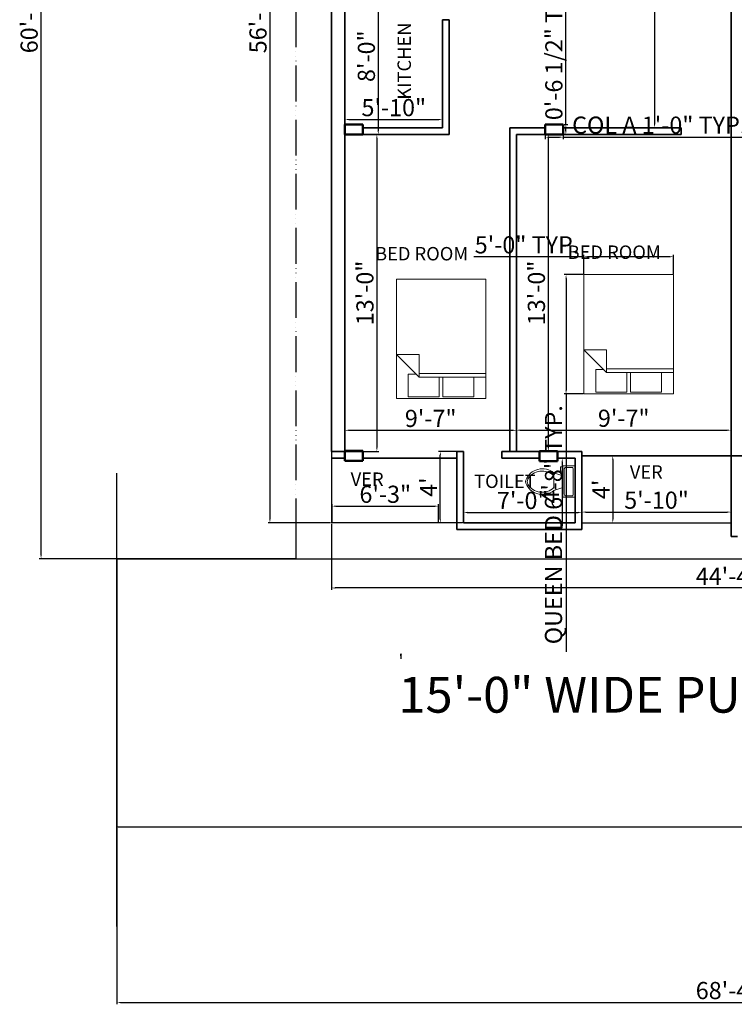
# Model space of a CAD drawing. Units: inches. Extents: x 2680 to 3617, y 1720 to 2823.
# Tile 1 of 4: x 2680 to 3159, y 1720 to 2380. Entities that reach past the tile are written whole.
import ezdxf

# ---------------------------------------------------------------- set-up
doc = ezdxf.new("R2010")
doc.units = ezdxf.units.IN
doc.linetypes.add('ACAD_ISO06W100', pattern=[36, 24, -3, 0, -3, 0, -3, 0, -3])
for name, color, linetype, lineweight in [('A-ANNO-DIMS', 2, 'Continuous', 18), ('A-ANNO-TEXT', 3, 'Continuous', 18), ('A-AREA-IDEN', 244, 'Continuous', 18), ('A-COLS', 1, 'Continuous', 50), ('A-FLOR', 7, 'Continuous', 25), ('A-FLOR-FIXT', 9, 'Continuous', 18), ('A-FURN', 8, 'Continuous', 18), ('A-WALL', 7, 'Continuous', 35), ('C-PROP', 6, 'ACAD_ISO06W100', 25), ('C-ROAD', 244, 'Continuous', 25)]:
    doc.layers.add(name, color=color, linetype=linetype, lineweight=lineweight)
doc.styles.get("Standard").update_dxf_attribs({"font": 'arial.ttf'})
doc.dimstyles.new('ISO-25', dxfattribs={"dimtxt": 11.5, "dimasz": 2.5, "dimexe": 1.25, "dimexo": 0.625, "dimtad": 1, "dimdec": 1, "dimlunit": 3, "dimtxsty": 'Standard', "dimcen": 2.5, "dimadec": 0, "dimazin": 0, "dimtfac": 1, "dimtdec": 1, "dimtmove": 0, "dimatfit": 3, "dimfxl": 1, "dimarcsym": 0})

# ---------------------------------------------------------------- blocks, each defined once
blk = doc.blocks.new('*D15')
at = {"layer": 'A-ANNO-DIMS', "color": 0, "lineweight": -2, "transparency": 16777216}
for p, q in [((2898.54, 2408), (2921.5, 2408)), ((2920.25, 2405.5), (2920.25, 2305.5)), ((2898.54, 2303), (2921.5, 2303))]:
    blk.add_line(p, q, dxfattribs=at)
at = {"layer": 'A-ANNO-DIMS', "color": 0, "lineweight": 70, "transparency": 16777216}
for points in [[(2919.83, 2405.5), (2920.66, 2405.5), (2920.25, 2408)], [(2919.83, 2305.5), (2920.66, 2305.5), (2920.25, 2303)]]:
    blk.add_solid(points, dxfattribs=at)
at = {"layer": 'Defpoints', "color": 0, "lineweight": 70, "transparency": 16777216}
for p in [(2897.91, 2408), (2897.91, 2303), (2920.25, 2303)]:
    blk.add_point(p, dxfattribs=at)
at = {"layer": 'A-ANNO-DIMS', "color": 0, "transparency": 16777216, "insert": (2913.75, 2355.5), "char_height": 11.5, "width": 30.5856, "attachment_point": 5, "rotation": 90}
blk.add_mtext('8\'-0"', dxfattribs=at)
blk = doc.blocks.new('*D17')
at = {"layer": 'A-ANNO-DIMS', "color": 0, "lineweight": -2, "transparency": 16777216}
for p, q in [((2897.91, 2310.27), (2897.91, 2314.28)), ((2900.41, 2313.03), (2960.91, 2313.03)), ((2963.41, 2308.13), (2963.41, 2314.28))]:
    blk.add_line(p, q, dxfattribs=at)
at = {"layer": 'A-ANNO-DIMS', "color": 0, "lineweight": 70, "transparency": 16777216}
for points in [[(2900.41, 2313.45), (2900.41, 2312.62), (2897.91, 2313.03)], [(2960.91, 2313.45), (2960.91, 2312.62), (2963.41, 2313.03)]]:
    blk.add_solid(points, dxfattribs=at)
at = {"layer": 'Defpoints', "color": 0, "lineweight": 70, "transparency": 16777216}
for p in [(2963.41, 2313.03), (2897.91, 2309.65), (2963.41, 2307.5)]:
    blk.add_point(p, dxfattribs=at)
at = {"layer": 'A-ANNO-DIMS', "color": 0, "transparency": 16777216, "insert": (2930.66, 2319.53), "char_height": 11.5, "attachment_point": 5}
blk.add_mtext('5\'-10"', dxfattribs=at)
blk = doc.blocks.new('*D18')
at = {"layer": 'A-ANNO-DIMS', "color": 0, "lineweight": -2, "transparency": 16777216}
for p, q in [((2898.54, 2303), (2920.56, 2303)), ((2919.31, 2300.5), (2919.31, 2093)), ((2898.52, 2090.5), (2920.56, 2090.5))]:
    blk.add_line(p, q, dxfattribs=at)
at = {"layer": 'A-ANNO-DIMS', "color": 0, "lineweight": 70, "transparency": 16777216}
for points in [[(2918.89, 2300.5), (2919.72, 2300.5), (2919.31, 2303)], [(2918.89, 2093), (2919.72, 2093), (2919.31, 2090.5)]]:
    blk.add_solid(points, dxfattribs=at)
at = {"layer": 'Defpoints', "color": 0, "lineweight": 70, "transparency": 16777216}
for p in [(2897.91, 2303), (2897.9, 2090.5), (2919.31, 2090.5)]:
    blk.add_point(p, dxfattribs=at)
at = {"layer": 'A-ANNO-DIMS', "color": 0, "transparency": 16777216, "insert": (2912.81, 2196.75), "char_height": 11.5, "attachment_point": 5, "rotation": 90}
blk.add_mtext('13\'-0"', dxfattribs=at)
blk = doc.blocks.new('*D19')
at = {"layer": 'A-ANNO-DIMS', "color": 0, "lineweight": -2, "transparency": 16777216}
for p, q in [((2897.91, 2091.13), (2897.91, 2105.87)), ((2900.41, 2104.62), (3010.41, 2104.62)), ((3012.91, 2091.13), (3012.91, 2105.87))]:
    blk.add_line(p, q, dxfattribs=at)
at = {"layer": 'A-ANNO-DIMS', "color": 0, "lineweight": 70, "transparency": 16777216}
for points in [[(2900.41, 2105.04), (2900.41, 2104.21), (2897.91, 2104.62)], [(3010.41, 2105.04), (3010.41, 2104.21), (3012.91, 2104.62)]]:
    blk.add_solid(points, dxfattribs=at)
at = {"layer": 'Defpoints', "color": 0, "lineweight": 70, "transparency": 16777216}
for p in [(3012.91, 2104.62), (2897.91, 2090.5), (3012.91, 2090.5)]:
    blk.add_point(p, dxfattribs=at)
at = {"layer": 'A-ANNO-DIMS', "color": 0, "transparency": 16777216, "insert": (2955.41, 2111.12), "char_height": 11.5, "attachment_point": 5}
blk.add_mtext('9\'-7"', dxfattribs=at)
blk = doc.blocks.new('*D20')
at = {"layer": 'A-ANNO-DIMS', "color": 0, "lineweight": -2, "transparency": 16777216}
for p, q in [((3013.56, 2303), (3035.58, 2303)), ((3034.33, 2300.5), (3034.33, 2093)), ((3013.54, 2090.5), (3035.58, 2090.5))]:
    blk.add_line(p, q, dxfattribs=at)
at = {"layer": 'A-ANNO-DIMS', "color": 0, "lineweight": 70, "transparency": 16777216}
for points in [[(3033.91, 2300.5), (3034.74, 2300.5), (3034.33, 2303)], [(3033.91, 2093), (3034.74, 2093), (3034.33, 2090.5)]]:
    blk.add_solid(points, dxfattribs=at)
at = {"layer": 'Defpoints', "color": 0, "lineweight": 70, "transparency": 16777216}
for p in [(3012.93, 2303), (3012.91, 2090.5), (3034.33, 2090.5)]:
    blk.add_point(p, dxfattribs=at)
at = {"layer": 'A-ANNO-DIMS', "color": 0, "transparency": 16777216, "insert": (3027.83, 2196.75), "char_height": 11.5, "attachment_point": 5, "rotation": 90}
blk.add_mtext('13\'-0"', dxfattribs=at)
blk = doc.blocks.new('*D24')
at = {"layer": 'A-ANNO-DIMS', "color": 0, "lineweight": -2, "transparency": 16777216}
for p, q in [((3012.91, 2091.23), (3012.91, 2105.97)), ((3015.41, 2104.72), (3154.41, 2104.72)), ((3156.91, 2091.23), (3156.91, 2105.97))]:
    blk.add_line(p, q, dxfattribs=at)
at = {"layer": 'A-ANNO-DIMS', "color": 0, "lineweight": 70, "transparency": 16777216}
for points in [[(3015.41, 2105.14), (3015.41, 2104.31), (3012.91, 2104.72)], [(3154.41, 2105.14), (3154.41, 2104.31), (3156.91, 2104.72)]]:
    blk.add_solid(points, dxfattribs=at)
at = {"layer": 'Defpoints', "color": 0, "lineweight": 70, "transparency": 16777216}
for p in [(3156.91, 2104.72), (3012.91, 2090.6), (3156.91, 2090.6)]:
    blk.add_point(p, dxfattribs=at)
at = {"layer": 'A-ANNO-DIMS', "color": 0, "transparency": 16777216, "insert": (3084.91, 2111.22), "char_height": 11.5, "attachment_point": 5}
blk.add_mtext('9\'-7"', dxfattribs=at)
blk = doc.blocks.new('*D25')
at = {"layer": 'A-ANNO-DIMS', "color": 0, "lineweight": -2, "transparency": 16777216}
for p, q in [((3082.04, 2521.5), (3106.78, 2521.5)), ((3105.53, 2519), (3105.53, 2310)), ((3084.49, 2307.5), (3106.78, 2307.5))]:
    blk.add_line(p, q, dxfattribs=at)
at = {"layer": 'A-ANNO-DIMS', "color": 0, "lineweight": 70, "transparency": 16777216}
for points in [[(3105.11, 2519), (3105.94, 2519), (3105.53, 2521.5)], [(3105.11, 2310), (3105.94, 2310), (3105.53, 2307.5)]]:
    blk.add_solid(points, dxfattribs=at)
at = {"layer": 'Defpoints', "color": 0, "lineweight": 70, "transparency": 16777216}
for p in [(3081.41, 2521.5), (3083.86, 2307.5), (3105.53, 2307.5)]:
    blk.add_point(p, dxfattribs=at)
at = {"layer": 'A-ANNO-DIMS', "color": 0, "transparency": 16777216, "insert": (3099.03, 2414.5), "char_height": 11.5, "attachment_point": 5, "rotation": 90}
blk.add_mtext('17\'-10"', dxfattribs=at)
blk = doc.blocks.new('*D28')
at = {"layer": 'A-ANNO-DIMS', "color": 0, "lineweight": -2, "transparency": 16777216}
for p, q in [((2976.79, 2090.5), (2960.62, 2090.5)), ((2961.87, 2045), (2961.87, 2088)), ((2976.79, 2042.5), (2960.62, 2042.5))]:
    blk.add_line(p, q, dxfattribs=at)
at = {"layer": 'A-ANNO-DIMS', "color": 0, "lineweight": 70, "transparency": 16777216}
for points in [[(2961.46, 2088), (2962.29, 2088), (2961.87, 2090.5)], [(2961.46, 2045), (2962.29, 2045), (2961.87, 2042.5)]]:
    blk.add_solid(points, dxfattribs=at)
at = {"layer": 'Defpoints', "color": 0, "lineweight": 70, "transparency": 16777216}
for p in [(2961.87, 2090.5), (2977.41, 2090.5), (2977.41, 2042.5)]:
    blk.add_point(p, dxfattribs=at)
at = {"layer": 'A-ANNO-DIMS', "color": 0, "transparency": 16777216, "insert": (2955.5, 2066.5), "char_height": 11.5, "attachment_point": 5, "rotation": 90}
blk.add_mtext("4'", dxfattribs=at)
blk = doc.blocks.new('*D29')
at = {"layer": 'A-ANNO-DIMS', "color": 0, "lineweight": -2, "transparency": 16777216}
for p, q in [((2889.28, 2043.13), (2889.28, 2055)), ((2891.78, 2053.75), (2958.12, 2053.75)), ((2960.62, 2043.13), (2960.62, 2055))]:
    blk.add_line(p, q, dxfattribs=at)
at = {"layer": 'A-ANNO-DIMS', "color": 0, "lineweight": 70, "transparency": 16777216}
for points in [[(2891.78, 2054.17), (2891.78, 2053.33), (2889.28, 2053.75)], [(2958.12, 2054.17), (2958.12, 2053.33), (2960.62, 2053.75)]]:
    blk.add_solid(points, dxfattribs=at)
at = {"layer": 'Defpoints', "color": 0, "lineweight": 70, "transparency": 16777216}
for p in [(2960.62, 2053.75), (2889.28, 2042.5), (2960.62, 2042.5)]:
    blk.add_point(p, dxfattribs=at)
at = {"layer": 'A-ANNO-DIMS', "color": 0, "transparency": 16777216, "insert": (2924.95, 2060.25), "char_height": 11.5, "attachment_point": 5}
blk.add_mtext('6\'-3"', dxfattribs=at)
blk = doc.blocks.new('*D30')
at = {"layer": 'A-ANNO-DIMS', "color": 0, "lineweight": -2, "transparency": 16777216}
for p, q in [((3051.79, 2086), (3042.43, 2086)), ((3043.68, 2083.5), (3043.68, 2040.5)), ((3051.79, 2038), (3042.43, 2038))]:
    blk.add_line(p, q, dxfattribs=at)
at = {"layer": 'A-ANNO-DIMS', "color": 0, "lineweight": 70, "transparency": 16777216}
for points in [[(3043.26, 2083.5), (3044.09, 2083.5), (3043.68, 2086)], [(3043.26, 2040.5), (3044.09, 2040.5), (3043.68, 2038)]]:
    blk.add_solid(points, dxfattribs=at)
at = {"layer": 'Defpoints', "color": 0, "lineweight": 70, "transparency": 16777216}
for p in [(3052.41, 2086), (3043.68, 2038), (3052.41, 2038)]:
    blk.add_point(p, dxfattribs=at)
at = {"layer": 'A-ANNO-DIMS', "color": 0, "transparency": 16777216, "insert": (3037.3, 2062), "char_height": 11.5, "attachment_point": 5, "rotation": 90}
blk.add_mtext("4'", dxfattribs=at)
blk = doc.blocks.new('*D31')
at = {"layer": 'A-ANNO-DIMS', "color": 0, "lineweight": -2, "transparency": 16777216}
for p, q in [((3057.54, 2087.51), (3078.82, 2087.51)), ((3077.57, 2085.01), (3077.57, 2045)), ((3057.54, 2042.5), (3078.82, 2042.5))]:
    blk.add_line(p, q, dxfattribs=at)
at = {"layer": 'A-ANNO-DIMS', "color": 0, "lineweight": 70, "transparency": 16777216}
for points in [[(3077.15, 2085.01), (3077.98, 2085.01), (3077.57, 2087.51)], [(3077.15, 2045), (3077.98, 2045), (3077.57, 2042.5)]]:
    blk.add_solid(points, dxfattribs=at)
at = {"layer": 'Defpoints', "color": 0, "lineweight": 70, "transparency": 16777216}
for p in [(3056.91, 2087.51), (3056.91, 2042.5), (3077.57, 2042.5)]:
    blk.add_point(p, dxfattribs=at)
at = {"layer": 'A-ANNO-DIMS', "color": 0, "transparency": 16777216, "insert": (3071.19, 2065.01), "char_height": 11.5, "attachment_point": 5, "rotation": 90}
blk.add_mtext("4'", dxfattribs=at)
blk = doc.blocks.new('*D34')
at = {"layer": 'A-ANNO-DIMS', "color": 0, "lineweight": -2, "transparency": 16777216}
for p, q in [((2977.41, 2043.13), (2977.41, 2050.82)), ((2979.91, 2049.57), (3054.41, 2049.57)), ((3056.91, 2043.13), (3056.91, 2050.82))]:
    blk.add_line(p, q, dxfattribs=at)
at = {"layer": 'A-ANNO-DIMS', "color": 0, "lineweight": 70, "transparency": 16777216}
for points in [[(2979.91, 2049.98), (2979.91, 2049.15), (2977.41, 2049.57)], [(3054.41, 2049.98), (3054.41, 2049.15), (3056.91, 2049.57)]]:
    blk.add_solid(points, dxfattribs=at)
at = {"layer": 'Defpoints', "color": 0, "lineweight": 70, "transparency": 16777216}
for p in [(3056.91, 2049.57), (2977.41, 2042.5), (3056.91, 2042.5)]:
    blk.add_point(p, dxfattribs=at)
at = {"layer": 'A-ANNO-DIMS', "color": 0, "transparency": 16777216, "insert": (3017.16, 2056.06), "char_height": 11.5, "attachment_point": 5}
blk.add_mtext('7\'-0"', dxfattribs=at)
blk = doc.blocks.new('*D35')
at = {"layer": 'A-ANNO-DIMS', "color": 0, "lineweight": -2, "transparency": 16777216}
for p, q in [((3056.91, 2043.13), (3056.91, 2051.04)), ((3059.41, 2049.79), (3154.41, 2049.79)), ((3156.91, 2043.13), (3156.91, 2051.04))]:
    blk.add_line(p, q, dxfattribs=at)
at = {"layer": 'A-ANNO-DIMS', "color": 0, "lineweight": 70, "transparency": 16777216}
for points in [[(3059.41, 2050.2), (3059.41, 2049.37), (3056.91, 2049.79)], [(3154.41, 2050.2), (3154.41, 2049.37), (3156.91, 2049.79)]]:
    blk.add_solid(points, dxfattribs=at)
at = {"layer": 'Defpoints', "color": 0, "lineweight": 70, "transparency": 16777216}
for p in [(3156.91, 2049.79), (3056.91, 2042.5), (3156.91, 2042.5)]:
    blk.add_point(p, dxfattribs=at)
at = {"layer": 'A-ANNO-DIMS', "color": 0, "transparency": 16777216, "insert": (3106.91, 2056.28), "char_height": 11.5, "attachment_point": 5}
blk.add_mtext('5\'-10"', dxfattribs=at)
blk = doc.blocks.new('*D40')
at = {"layer": 'A-ANNO-DIMS', "color": 0, "lineweight": -2, "transparency": 16777216}
for p, q in [((2888.91, 2041.88), (2888.91, 1997.63)), ((3420.91, 2041.88), (3420.91, 1997.63)), ((3418.41, 1998.88), (2891.41, 1998.88))]:
    blk.add_line(p, q, dxfattribs=at)
at = {"layer": 'A-ANNO-DIMS', "color": 0, "lineweight": 70, "transparency": 16777216}
for points in [[(2891.41, 1999.29), (2891.41, 1998.46), (2888.91, 1998.88)], [(3418.41, 1999.29), (3418.41, 1998.46), (3420.91, 1998.88)]]:
    blk.add_solid(points, dxfattribs=at)
at = {"layer": 'Defpoints', "color": 0, "lineweight": 70, "transparency": 16777216}
for p in [(2888.91, 2042.5), (3420.91, 2042.5), (2888.91, 1998.88)]:
    blk.add_point(p, dxfattribs=at)
at = {"layer": 'A-ANNO-DIMS', "color": 0, "transparency": 16777216, "insert": (3154.91, 2005.25), "char_height": 11.5, "attachment_point": 5}
blk.add_mtext('44\'-4"', dxfattribs=at)
blk = doc.blocks.new('*D42')
at = {"layer": 'A-ANNO-DIMS', "color": 0, "lineweight": -2, "transparency": 16777216}
for p, q in [((2888.29, 2724.5), (2846.31, 2724.5)), ((2847.56, 2722), (2847.56, 2045)), ((2888.29, 2042.5), (2846.31, 2042.5))]:
    blk.add_line(p, q, dxfattribs=at)
at = {"layer": 'A-ANNO-DIMS', "color": 0, "lineweight": 70, "transparency": 16777216}
for points in [[(2847.14, 2722), (2847.98, 2722), (2847.56, 2724.5)], [(2847.14, 2045), (2847.98, 2045), (2847.56, 2042.5)]]:
    blk.add_solid(points, dxfattribs=at)
at = {"layer": 'Defpoints', "color": 0, "lineweight": 70, "transparency": 16777216}
for p in [(2888.91, 2724.5), (2847.56, 2042.5), (2888.91, 2042.5)]:
    blk.add_point(p, dxfattribs=at)
at = {"layer": 'A-ANNO-DIMS', "color": 0, "transparency": 16777216, "insert": (2841.06, 2383.5), "char_height": 11.5, "attachment_point": 5, "rotation": 90}
blk.add_mtext('56\'-10"', dxfattribs=at)
blk = doc.blocks.new('Bed - Queen')
for p, q in [((0, -80.00003), (0, 0)), ((0, 0), (59.99999, 0)), ((59.99999, 0), (59.99999, -80.00003)), ((7.99999, -1.2), (28.79998, -1.2)), ((7.99999, -14.4), (7.99999, -1.2)), ((28.79998, -1.2), (28.79998, -14.4)), ((31.19999, -1.2), (51.99999, -1.2)), ((31.19999, -14.4), (31.19999, -1.2)), ((51.99999, -1.2), (51.99999, -16.4)), ((0, -14.4), (44.8, -14.4)), ((44.8, -16.8), (0, -16.8)), ((59.99999, -29.6), (44.8, -14.4)), ((44.8, -14.4), (44.8, -29.6)), ((51.99999, -16.4), (46.79936, -16.4)), ((44.8, -29.6), (59.99999, -29.6)), ((59.99999, -80.00003), (0, -80.00003))]:
    blk.add_line(p, q)
blk = doc.blocks.new('Toilet - top')
for p, q in [((9.5, -6), (9.5, -2)), ((-10, -8.5), (-8, -8.5)), ((-10, -9.5), (-10, -8.5)), ((-7, -9.5), (-10, -9.5)), ((-8, -8.5), (-8, -8)), ((-7, -8), (-7, -9.5)), ((-4, -8), (-6, -14)), ((4, -8), (6, -14)), ((4, -14), (-4, -14))]:
    blk.add_line(p, q)
blk.add_lwpolyline([(10.5, -8), (10.5, 0), (-10.5, 0), (-10.5, -8)], close=True)
for points in [[(-9.5, -2), (-9.5, -6)], [(8.5, -1), (-8.5, -1)], [(-8.5, -7), (8.5, -7)]]:
    blk.add_lwpolyline(points)
for centre, radius, start, end in [((-8.62, -1.88), 0.884, 81.8699, 188.1301), ((-8.62, -6.12), 0.884, 171.8699, 278.1301), ((8.62, -1.88), 0.884, 351.8699, 98.1301), ((8.62, -6.12), 0.884, 261.8699, 8.1301), ((3.52, -21.58), 12.17, 141.46911, 247.97143), ((4.2, -21.82), 11.33, 136.36773, 238.94682), ((-3.52, -21.58), 12.17, 292.02843, 38.53071), ((-4.2, -21.82), 11.33, 301.05301, 43.63209), ((0, -27.88), 4, 245.73182, 294.26817), ((0, -29), 4, 254.86053, 285.13947)]:
    blk.add_arc(centre, radius, start, end)
blk = doc.blocks.new('COL-12X6P64')
for p, q in [((0, 0), (0, 6.64)), ((0, 6.64), (12, 6.64)), ((12, 6.64), (12, 0)), ((12, 0), (0, 0))]:
    blk.add_line(p, q)
blk = doc.blocks.new('*D54')
at = {"layer": 'A-ANNO-DIMS', "color": 0, "lineweight": -2, "transparency": 16777216}
for p, q in [((3057.61, 2209.02), (3044.98, 2209.02)), ((3046.23, 2206.52), (3046.23, 2131.52)), ((3057.61, 2129.02), (3044.98, 2129.02)), ((3046.23, 2129.02), (3046.23, 1956.1))]:
    blk.add_line(p, q, dxfattribs=at)
at = {"layer": 'A-ANNO-DIMS', "color": 0, "lineweight": 70, "transparency": 16777216}
for points in [[(3045.82, 2206.52), (3046.65, 2206.52), (3046.23, 2209.02)], [(3045.82, 2131.52), (3046.65, 2131.52), (3046.23, 2129.02)]]:
    blk.add_solid(points, dxfattribs=at)
at = {"layer": 'Defpoints', "color": 0, "lineweight": 70, "transparency": 16777216}
for p in [(3058.23, 2209.02), (3046.23, 2129.02), (3058.23, 2129.02)]:
    blk.add_point(p, dxfattribs=at)
at = {"layer": 'A-ANNO-DIMS', "color": 0, "transparency": 16777216, "insert": (3039.31, 2041.31), "char_height": 11.5, "attachment_point": 5, "rotation": 90}
blk.add_mtext('QUEEN BED 6\'-8" TYP.', dxfattribs=at)
blk = doc.blocks.new('*D55')
at = {"layer": 'A-ANNO-DIMS', "color": 0, "lineweight": -2, "transparency": 16777216}
for p, q in [((3058.23, 2221.02), (2984.39, 2221.02)), ((3058.23, 2209.64), (3058.23, 2222.27)), ((3115.73, 2221.02), (3060.73, 2221.02)), ((3118.23, 2209.64), (3118.23, 2222.27))]:
    blk.add_line(p, q, dxfattribs=at)
at = {"layer": 'A-ANNO-DIMS', "color": 0, "lineweight": 70, "transparency": 16777216}
for points in [[(3060.73, 2221.43), (3060.73, 2220.6), (3058.23, 2221.02)], [(3115.73, 2221.43), (3115.73, 2220.6), (3118.23, 2221.02)]]:
    blk.add_solid(points, dxfattribs=at)
at = {"layer": 'Defpoints', "color": 0, "lineweight": 70, "transparency": 16777216}
for p in [(3058.23, 2221.02), (3058.23, 2209.02), (3118.23, 2209.02)]:
    blk.add_point(p, dxfattribs=at)
at = {"layer": 'A-ANNO-DIMS', "color": 0, "transparency": 16777216, "insert": (3020.06, 2227.51), "char_height": 11.5, "attachment_point": 5}
blk.add_mtext('5\'-0" TYP.', dxfattribs=at)
blk = doc.blocks.new('*D58')
at = {"layer": 'A-ANNO-DIMS', "color": 0, "lineweight": -2, "transparency": 16777216}
for p, q in [((3032.31, 2302.38), (3032.31, 2299.95)), ((3034.81, 2301.2), (3041.81, 2301.2)), ((3044.31, 2302.38), (3044.31, 2299.95)), ((3044.31, 2301.2), (3170.7, 2301.2))]:
    blk.add_line(p, q, dxfattribs=at)
at = {"layer": 'A-ANNO-DIMS', "color": 0, "lineweight": 70, "transparency": 16777216}
for points in [[(3034.81, 2301.62), (3034.81, 2300.79), (3032.31, 2301.2)], [(3041.81, 2301.62), (3041.81, 2300.79), (3044.31, 2301.2)]]:
    blk.add_solid(points, dxfattribs=at)
at = {"layer": 'Defpoints', "color": 0, "lineweight": 70, "transparency": 16777216}
for p in [(3032.31, 2303), (3044.31, 2303), (3044.31, 2301.2)]:
    blk.add_point(p, dxfattribs=at)
at = {"layer": 'A-ANNO-DIMS', "color": 0, "transparency": 16777216, "insert": (3108.75, 2307.78), "char_height": 11.5, "attachment_point": 5}
blk.add_mtext('COL A 1\'-0" TYP.', dxfattribs=at)
blk = doc.blocks.new('*D59')
at = {"layer": 'A-ANNO-DIMS', "color": 0, "lineweight": -2, "transparency": 16777216}
for p, q in [((3046.11, 2309.65), (3046.11, 2410.29)), ((3044.93, 2309.65), (3047.36, 2309.65)), ((3046.11, 2305.5), (3046.11, 2307.15)), ((3044.93, 2303), (3047.36, 2303))]:
    blk.add_line(p, q, dxfattribs=at)
at = {"layer": 'A-ANNO-DIMS', "color": 0, "lineweight": 70, "transparency": 16777216}
for points in [[(3045.69, 2307.15), (3046.52, 2307.15), (3046.11, 2309.65)], [(3045.69, 2305.5), (3046.52, 2305.5), (3046.11, 2303)]]:
    blk.add_solid(points, dxfattribs=at)
at = {"layer": 'Defpoints', "color": 0, "lineweight": 70, "transparency": 16777216}
for p in [(3044.31, 2309.65), (3046.11, 2309.65), (3044.31, 2303)]:
    blk.add_point(p, dxfattribs=at)
at = {"layer": 'A-ANNO-DIMS', "color": 0, "transparency": 16777216, "insert": (3039.54, 2361.22), "char_height": 11.5, "attachment_point": 5, "rotation": 90}
blk.add_mtext('0\'-6 1/2" TYP.', dxfattribs=at)
blk = doc.blocks.new('*D69')
at = {"layer": 'A-ANNO-DIMS', "color": 0, "lineweight": -2, "transparency": 16777216}
for p, q in [((2864.29, 2748.5), (2692.76, 2748.5)), ((2694.01, 2021), (2694.01, 2746)), ((2864.29, 2018.5), (2692.76, 2018.5))]:
    blk.add_line(p, q, dxfattribs=at)
at = {"layer": 'A-ANNO-DIMS', "color": 0, "lineweight": 70, "transparency": 16777216}
for points in [[(2693.6, 2746), (2694.43, 2746), (2694.01, 2748.5)], [(2693.6, 2021), (2694.43, 2021), (2694.01, 2018.5)]]:
    blk.add_solid(points, dxfattribs=at)
at = {"layer": 'Defpoints', "color": 0, "lineweight": 70, "transparency": 16777216}
for p in [(2694.01, 2748.5), (2864.91, 2748.5), (2864.91, 2018.5)]:
    blk.add_point(p, dxfattribs=at)
at = {"layer": 'A-ANNO-DIMS', "color": 0, "transparency": 16777216, "insert": (2687.52, 2383.5), "char_height": 11.5, "attachment_point": 5, "rotation": 90}
blk.add_mtext('60\'-10"', dxfattribs=at)
blk = doc.blocks.new('*D70')
at = {"layer": 'A-ANNO-DIMS', "color": 0, "lineweight": -2, "transparency": 16777216}
for p, q in [((2744.91, 1837.88), (2744.91, 1719.69)), ((3564.91, 1837.88), (3564.91, 1719.69)), ((2747.41, 1720.94), (3562.41, 1720.94))]:
    blk.add_line(p, q, dxfattribs=at)
at = {"layer": 'A-ANNO-DIMS', "color": 0, "lineweight": 70, "transparency": 16777216}
for points in [[(2747.41, 1721.36), (2747.41, 1720.52), (2744.91, 1720.94)], [(3562.41, 1721.36), (3562.41, 1720.52), (3564.91, 1720.94)]]:
    blk.add_solid(points, dxfattribs=at)
at = {"layer": 'Defpoints', "color": 0, "lineweight": 70, "transparency": 16777216}
for p in [(2744.91, 1838.5), (3564.91, 1838.5), (3564.91, 1720.94)]:
    blk.add_point(p, dxfattribs=at)
at = {"layer": 'A-ANNO-DIMS', "color": 0, "transparency": 16777216, "insert": (3154.91, 1727.44), "char_height": 11.5, "attachment_point": 5}
blk.add_mtext('68\'-4"', dxfattribs=at)

msp = doc.modelspace()

# ---------------------------------------------------------------- linework, layer by layer
at = {"layer": 'A-FLOR'}
for p, q in [((2888.91, 2090.5), (2888.91, 2042.5)), ((2972.91, 2042.5), (2888.91, 2042.5)), ((3056.91, 2042.5), (3156.91, 2042.5))]:
    msp.add_line(p, q, dxfattribs=at)
at = {"layer": 'A-WALL'}
for p, q in [((2888.91, 2090.5), (2888.91, 2724.5)), ((2897.91, 2090.5), (2897.91, 2715.5)), ((3156.91, 2521.5), (3156.91, 2042.5)), ((2963.41, 2307.5), (2963.41, 2379.98)), ((2963.41, 2379.98), (2967.91, 2379.98)), ((2967.91, 2303), (2967.91, 2379.98)), ((2909.91, 2307.5), (2963.41, 2307.5)), ((3008.41, 2090.5), (3008.41, 2307.5)), ((3008.41, 2307.5), (3032.31, 2307.5)), ((3044.31, 2307.5), (3123.41, 2307.5)), ((3123.41, 2303), (3123.41, 2307.5)), ((2897.91, 2303), (2967.91, 2303)), ((3012.91, 2090.5), (3012.91, 2303)), ((3012.91, 2303), (3123.41, 2303)), ((2897.91, 2090.5), (2888.91, 2090.5)), ((2972.91, 2038), (2972.91, 2090.5)), ((2977.41, 2090.5), (2972.91, 2090.5)), ((2977.41, 2042.5), (2977.41, 2090.5)), ((3003.25, 2090.5), (3003.25, 2086)), ((3056.91, 2090.5), (3003.25, 2090.5)), ((3056.91, 2038), (3056.91, 2090.5)), ((3056.91, 2087.51), (3252.91, 2087.51)), ((2897.9, 2086), (2888.91, 2086)), ((2972.91, 2086), (2909.9, 2086)), ((3028.48, 2086), (3003.25, 2086)), ((3052.41, 2086), (3040.48, 2086)), ((3052.41, 2042.5), (3052.41, 2086)), ((3052.41, 2042.5), (2977.41, 2042.5)), ((3156.91, 2042.5), (3156.91, 2033.5)), ((3056.91, 2038), (2972.91, 2038)), ((3156.91, 2033.5), (3161.31, 2033.5))]:
    msp.add_line(p, q, dxfattribs=at)
at = {"layer": 'C-PROP'}
for p, q in [((2864.91, 2748.5), (2864.91, 2042.5)), ((2864.91, 2042.5), (2864.91, 2018.5))]:
    msp.add_line(p, q, dxfattribs=at)
at = {"layer": 'C-ROAD'}
for p, q in [((2744.91, 2018.5), (2744.91, 2075.96)), ((2744.91, 2018.5), (2744.91, 1838.5)), ((2864.91, 2018.5), (2804.91, 2018.5))]:
    msp.add_line(p, q, dxfattribs=at)
for points in [[(2744.91, 1771.84), (2744.91, 1838.5), (2744.91, 2018.5), (2804.91, 2018.5), (2984.91, 2018.5), (3444.91, 2018.5), (3504.91, 2018.5), (3564.91, 2018.5), (3564.91, 2075.96)], [(3564.91, 1771.84), (3564.91, 2018.5), (3564.91, 1838.5), (3504.91, 1838.5), (3444.91, 1838.5), (2984.91, 1838.5), (2804.91, 1838.5), (2744.91, 1838.5)]]:
    msp.add_lwpolyline(points, dxfattribs=at)

# ---------------------------------------------------------------- block references
at = {"layer": 'A-COLS'}
for p in [(2897.91, 2303), (3032.31, 2303), (2897.9, 2084.26), (3028.48, 2083.96)]:
    msp.add_blockref('COL-12X6P64', p, dxfattribs=at)
at = {"layer": 'A-FLOR-FIXT', "rotation": 270}
msp.add_blockref('Toilet - top', (3052.07, 2070.19), dxfattribs=at)
at = {"layer": 'A-FURN', "rotation": 180}
for p in [(2992.38, 2125.92), (3118.23, 2129.02)]:
    msp.add_blockref('Bed - Queen', p, dxfattribs=at)

# ---------------------------------------------------------------- texts
at = {"layer": 'A-ANNO-TEXT', "insert": (2933.78, 1954.28), "char_height": 9, "attachment_point": 1}
msp.add_mtext_dynamic_manual_height_columns('\'\\P{\\H2.66667x;15\'-0" WIDE PUCCA ROAD}', width=461.2944, gutter_width=12.5, heights=[0], dxfattribs=at)
at = {"layer": 'A-AREA-IDEN', "insert": (2933.16, 2326.33), "char_height": 9, "attachment_point": 1, "rotation": 90}
msp.add_mtext_dynamic_manual_height_columns('{KITCHEN}', width=87.2951, gutter_width=12.5, heights=[0], dxfattribs=at)
at = {"layer": 'A-AREA-IDEN', "char_height": 9, "attachment_point": 1}
for s, insert in [('{BED ROOM}', (2918.12, 2227.54)), ('{BED ROOM}', (3047.3, 2228.57)), ('{VER}', (3089, 2081.17)), ('{VER}', (2901.74, 2076.33)), ('{TOILET}', (2984.56, 2074.94))]:
    msp.add_mtext_dynamic_manual_height_columns(s, width=87.2951, gutter_width=12.5, heights=[0], dxfattribs=dict(at, insert=insert))

# ---------------------------------------------------------------- dimensions: what is measured, and where the dimension line sits
at = {"layer": 'A-ANNO-DIMS'}
for base, p1, p2, override, picture, middle in [((2694.01, 2748.5), (2864.91, 2018.5), (2864.91, 2748.5), {"dimdec": 1, "dimlfac": 1, "dimrnd": 0, "dimzin": 1, "dimdsep": 46, "dimlunit": 4, "dimfrac": 2}, '*D69', (2687.52, 2383.5)), ((2847.56, 2042.5), (2888.91, 2724.5), (2888.91, 2042.5), {"dimclrd": 0, "dimclre": 0, "dimclrt": 0}, '*D42', (2841.06, 2383.5)), ((3105.53, 2307.5), (3081.41, 2521.5), (3083.86, 2307.5), {"dimclrd": 0, "dimclre": 0, "dimclrt": 0}, '*D25', (3099.03, 2414.5)), ((2961.87, 2090.5), (2977.41, 2042.5), (2977.41, 2090.5), {"dimclrd": 0, "dimclre": 0, "dimclrt": 0}, '*D28', (2955.5, 2066.5)), ((3043.68, 2038), (3052.41, 2086), (3052.41, 2038), {"dimclrd": 0, "dimclre": 0, "dimclrt": 0}, '*D30', (3037.3, 2062))]:
    dim = msp.add_linear_dim(base=base, p1=p1, p2=p2, angle=90, dimstyle='ISO-25', override=override, dxfattribs=at)
    dim.commit()
    dim.dimension.update_dxf_attribs({"geometry": picture, "text_midpoint": middle})
for base, p1, p2, angle, text, override, picture, middle in [((3046.1082, 2309.6469), (3044.3082, 2303.0039), (3044.3082, 2309.6469), 90, '<> TYP.', {"dimdec": 1, "dimlfac": 1, "dimrnd": 0, "dimzin": 1, "dimdsep": 46, "dimlunit": 4, "dimfrac": 2}, '*D59', (3039.5371, 2361.2194)), ((2920.25, 2303), (2897.91, 2408), (2897.91, 2303), 90, '8\'-0"', {"dimclrd": 0, "dimclre": 0, "dimclrt": 0}, '*D15', (2913.75, 2355.5)), ((2919.31, 2090.5), (2897.91, 2303), (2897.9, 2090.5), 90, '13\'-0"', {"dimclrd": 0, "dimclre": 0, "dimclrt": 0}, '*D18', (2912.81, 2196.75)), ((3034.33, 2090.5), (3012.93, 2303), (3012.91, 2090.5), 90, '13\'-0"', {"dimclrd": 0, "dimclre": 0, "dimclrt": 0}, '*D20', (3027.83, 2196.75)), ((3058.23, 2221.02), (3118.23, 2209.02), (3058.23, 2209.02), 180, '<> TYP.', {"dimdec": 1, "dimlfac": 1, "dimrnd": 0, "dimzin": 1, "dimdsep": 46, "dimlunit": 4, "dimfrac": 2}, '*D55', (3020.06, 2227.51)), ((3046.23, 2129.02), (3058.23, 2209.02), (3058.23, 2129.02), 270, 'QUEEN BED <> TYP.', {"dimdec": 1, "dimlfac": 1, "dimrnd": 0, "dimzin": 1, "dimdsep": 46, "dimlunit": 4, "dimfrac": 2}, '*D54', (3039.31, 2041.31)), ((3077.57, 2042.5), (3056.91, 2087.51), (3056.91, 2042.5), 90, "4'", {"dimclrd": 0, "dimclre": 0, "dimclrt": 0}, '*D31', (3071.19, 2065.01))]:
    dim = msp.add_linear_dim(base=base, p1=p1, p2=p2, angle=angle, text=text, dimstyle='ISO-25', override=override, dxfattribs=at)
    dim.commit()
    dim.dimension.update_dxf_attribs({"geometry": picture, "text_midpoint": middle})
for base, p1, p2, text, override, picture, middle in [((3044.31, 2301.2), (3032.31, 2303), (3044.31, 2303), 'COL A <> TYP.', {"dimdec": 1, "dimlfac": 1, "dimrnd": 0, "dimzin": 1, "dimdsep": 46, "dimlunit": 4, "dimfrac": 2}, '*D58', (3108.75, 2307.78)), ((2963.41, 2313.03), (2897.91, 2309.65), (2963.41, 2307.5), '5\'-10"', {"dimclrd": 0, "dimclre": 0, "dimclrt": 0}, '*D17', (2930.66, 2319.53)), ((3156.91, 2104.72), (3012.91, 2090.6), (3156.91, 2090.6), '9\'-7"', {"dimclrd": 0, "dimclre": 0, "dimclrt": 0}, '*D24', (3084.91, 2111.22)), ((2960.62, 2053.75), (2889.28, 2042.5), (2960.62, 2042.5), '6\'-3"', {"dimclrd": 0, "dimclre": 0, "dimclrt": 0}, '*D29', (2924.95, 2060.25)), ((3056.91, 2049.57), (2977.41, 2042.5), (3056.91, 2042.5), '7\'-0"', {"dimclrd": 0, "dimclre": 0, "dimclrt": 0}, '*D34', (3017.16, 2056.06)), ((3156.91, 2049.79), (3056.91, 2042.5), (3156.91, 2042.5), '5\'-10"', {"dimclrd": 0, "dimclre": 0, "dimclrt": 0}, '*D35', (3106.91, 2056.28))]:
    dim = msp.add_linear_dim(base=base, p1=p1, p2=p2, text=text, dimstyle='ISO-25', override=override, dxfattribs=at)
    dim.commit()
    dim.dimension.update_dxf_attribs({"geometry": picture, "text_midpoint": middle})
for base, p1, p2, override, picture, middle in [((3012.91, 2104.62), (2897.91, 2090.5), (3012.91, 2090.5), {"dimclrd": 0, "dimclre": 0, "dimclrt": 0}, '*D19', (2955.41, 2111.12)), ((2888.91, 1998.88), (3420.91, 2042.5), (2888.91, 2042.5), {"dimclrd": 0, "dimclre": 0, "dimclrt": 0}, '*D40', (3154.91, 2005.25)), ((3564.91, 1720.94), (2744.91, 1838.5), (3564.91, 1838.5), {"dimdec": 1, "dimlfac": 1, "dimrnd": 0, "dimzin": 1, "dimdsep": 46, "dimlunit": 4, "dimfrac": 2}, '*D70', (3154.91, 1727.44))]:
    dim = msp.add_linear_dim(base=base, p1=p1, p2=p2, dimstyle='ISO-25', override=override, dxfattribs=at)
    dim.commit()
    dim.dimension.update_dxf_attribs({"geometry": picture, "text_midpoint": middle})

doc.saveas('drawing.dxf')
